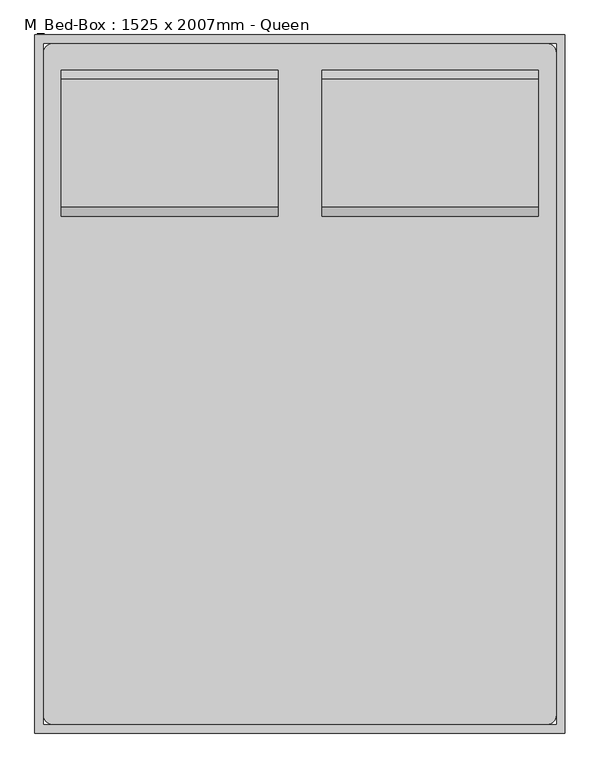
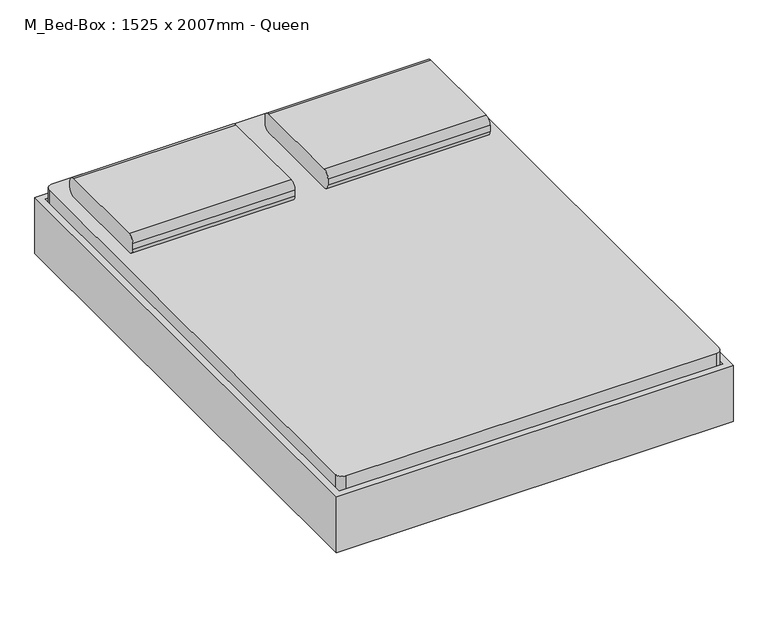
"""IFC4 building model written with IfcOpenShell, lengths in millimetres: furniture geometry, M_Bed-Box : 1525 x 2007mm - Queen."""

from ifc_helpers import new_model, si_unit, point, frame, frame_2d, origin, place, context, project, spatial, polyline, circle_curve, trimmed, segment, composite_curve, outline, extrude, source, transform, mapped, element, save
from ifc_brep_helpers import plane_surface, cylinder_surface, revolved_surface, advanced_brep


def m_bed_box_1525_x_2007mm_queen_e2603687(model_context):
    return source(origin(), model_context, "Body", "SolidModel", [
        extrude(outline(composite_curve([segment(polyline([(642.0704918, 406.4), (273.7704918, 406.4)]), True, "CONTINUOUS"), segment(trimmed(circle_curve(frame_2d((273.7704918, 431.8)), 25.4), [point((273.7704918, 406.4))], [point((248.3704918, 431.8))], False, "CARTESIAN"), True, "CONTINUOUS"), segment(polyline([(248.3704918, 431.8), (248.3704918, 457.2)]), True, "CONTINUOUS"), segment(trimmed(circle_curve(frame_2d((273.7704918, 457.2)), 25.4), [point((248.3704918, 457.2))], [point((273.7704918, 482.6))], False, "CARTESIAN"), True, "CONTINUOUS"), segment(polyline([(273.7704918, 482.6), (642.0704918, 482.6)]), True, "CONTINUOUS"), segment(trimmed(circle_curve(frame_2d((642.0704918, 457.2)), 25.4), [point((642.0704918, 482.6))], [point((667.4704918, 457.2))], False, "CARTESIAN"), True, "CONTINUOUS"), segment(polyline([(667.4704918, 457.2), (667.4704918, 431.8)]), True, "CONTINUOUS"), segment(trimmed(circle_curve(frame_2d((642.0704918, 431.8)), 25.4), [point((667.4704918, 431.8))], [point((642.0704918, 406.4))], False, "CARTESIAN"), True, "CONTINUOUS")], self_intersect=False)), frame((402.652459, 0.0, 0.0), z_axis=(1.0, 0.0, 0.0), x_axis=(0.0, 1.0, 0.0)), (0.0, 0.0, 1.0), 622.8),
        extrude(outline(composite_curve([segment(polyline([(642.0704918, 406.4), (273.7704918, 406.4)]), True, "CONTINUOUS"), segment(trimmed(circle_curve(frame_2d((273.7704918, 431.8)), 25.4), [point((273.7704918, 406.4))], [point((248.3704918, 431.8))], False, "CARTESIAN"), True, "CONTINUOUS"), segment(polyline([(248.3704918, 431.8), (248.3704918, 457.2)]), True, "CONTINUOUS"), segment(trimmed(circle_curve(frame_2d((273.7704918, 457.2)), 25.4), [point((248.3704918, 457.2))], [point((273.7704918, 482.6))], False, "CARTESIAN"), True, "CONTINUOUS"), segment(polyline([(273.7704918, 482.6), (642.0704918, 482.6)]), True, "CONTINUOUS"), segment(trimmed(circle_curve(frame_2d((642.0704918, 457.2)), 25.4), [point((642.0704918, 482.6))], [point((667.4704918, 457.2))], False, "CARTESIAN"), True, "CONTINUOUS"), segment(polyline([(667.4704918, 457.2), (667.4704918, 431.8)]), True, "CONTINUOUS"), segment(trimmed(circle_curve(frame_2d((642.0704918, 431.8)), 25.4), [point((667.4704918, 431.8))], [point((642.0704918, 406.4))], False, "CARTESIAN"), True, "CONTINUOUS")], self_intersect=False)), frame((-347.147541, 0.0, 0.0), z_axis=(1.0, 0.0, 0.0), x_axis=(0.0, 1.0, 0.0)), (0.0, 0.0, 1.0), 622.8),
        advanced_brep(
        [(-397.6231784, 515.0704918, 177.8), (-397.6231784, 438.8704918, 177.8), (-397.6231784, 438.8704918, 196.85), (-397.6231784, 515.0704918, 196.85), (-346.8231784, 515.0704918, 177.8), (-346.8231784, 438.8704918, 177.8), (-334.6869899, 438.8704918, 196.85), (-334.6869899, 515.0704918, 196.85), (-270.7523099, 515.0704918, 14.6654962), (-270.7523099, 438.8704918, 14.6654962), (-253.4871466, 438.8704918, 22.716374), (-253.4871466, 515.0704918, 22.716374), (-247.7320921, 438.8704918, 0.0), (-247.7320921, 515.0704918, 0.0), (-247.7320921, 438.8704918, 19.05), (-247.7320921, 515.0704918, 19.05), (-169.1195862, 515.0704918, 0.0), (-169.1195862, 438.8704918, 0.0), (-169.1195862, 438.8704918, 19.05), (-169.1195862, 515.0704918, 19.05), (-156.4195862, 438.8704918, 3.4029547), (-156.4195862, 515.0704918, 3.4029547), (-165.9445862, 438.8704918, 19.9007387), (-165.9445862, 515.0704918, 19.9007387), (-96.322541, 515.0704918, 38.1), (-96.322541, 438.8704918, 38.1), (-101.4269731, 438.8704918, 57.15), (-101.4269731, 515.0704918, 57.15), (774.9518216, 515.0704918, 38.1), (774.9518216, 438.8704918, 38.1), (780.0562537, 438.8704918, 57.15), (780.0562537, 515.0704918, 57.15), (835.0488669, 515.0704918, 3.4029547), (835.0488669, 438.8704918, 3.4029547), (844.5738669, 438.8704918, 19.9007387), (844.5738669, 515.0704918, 19.9007387), (847.7488669, 438.8704918, 0.0), (847.7488669, 515.0704918, 0.0), (847.7488669, 438.8704918, 19.05), (847.7488669, 515.0704918, 19.05), (926.3613728, 515.0704918, 0.0), (926.3613728, 438.8704918, 0.0), (926.3613728, 438.8704918, 19.05), (926.3613728, 515.0704918, 19.05), (949.3815906, 438.8704918, 14.6654962), (949.3815906, 515.0704918, 14.6654962), (932.1164272, 438.8704918, 22.716374), (932.1164272, 515.0704918, 22.716374), (1025.452459, 515.0704918, 177.8), (1025.452459, 438.8704918, 177.8), (1013.3162705, 438.8704918, 196.85), (1013.3162705, 515.0704918, 196.85), (1076.252459, 515.0704918, 177.8), (1076.252459, 515.0704918, 196.85), (1076.252459, 438.8704918, 196.85), (1076.252459, 438.8704918, 177.8)],
        [
            (0, 1),
            (1, 2),
            (2, 3),
            (3, 0),
            (0, 4),
            (4, 5),
            (5, 1),
            (5, 6),
            (6, 2),
            (6, 7),
            (7, 3),
            (7, 4),
            (4, 8),
            (8, 9),
            (9, 5),
            (9, 10),
            (10, 6),
            (10, 11),
            (11, 7),
            (11, 8),
            (12, 9, circle_curve(frame((-247.7320921, 438.8704918, 25.4), z_axis=(0.0, 1.0, 0.0), x_axis=(-0.906307787036649, 0.0, -0.4226182617407015)), 25.4)),
            (8, 13, circle_curve(frame((-247.7320921, 515.0704918, 25.4), z_axis=(0.0, -1.0, 0.0), x_axis=(-0.906307787036649, 0.0, -0.4226182617407015)), 25.4)),
            (13, 12),
            (14, 10, circle_curve(frame((-247.7320921, 438.8704918, 25.4), z_axis=(0.0, 1.0, 0.0), x_axis=(-0.906307787036649, 0.0, -0.4226182617407015)), 6.35)),
            (12, 14),
            (15, 11, circle_curve(frame((-247.7320921, 515.0704918, 25.4), z_axis=(0.0, 1.0, 0.0), x_axis=(-0.906307787036649, 0.0, -0.4226182617407015)), 6.35)),
            (14, 15),
            (15, 13),
            (13, 16),
            (16, 17),
            (17, 12),
            (17, 18),
            (18, 14),
            (18, 19),
            (19, 15),
            (19, 16),
            (20, 17, circle_curve(frame((-169.1195862, 438.8704918, 25.4), z_axis=(0.0, 1.0, 0.0), x_axis=(0.0, 0.0, -1.0)), 25.4)),
            (16, 21, circle_curve(frame((-169.1195862, 515.0704918, 25.4), z_axis=(0.0, -1.0, 0.0), x_axis=(0.0, 0.0, -1.0)), 25.4)),
            (21, 20),
            (22, 18, circle_curve(frame((-169.1195862, 438.8704918, 25.4), z_axis=(0.0, 1.0, 0.0), x_axis=(0.0, 0.0, -1.0)), 6.35)),
            (20, 22),
            (23, 19, circle_curve(frame((-169.1195862, 515.0704918, 25.4), z_axis=(0.0, 1.0, 0.0), x_axis=(0.0, 0.0, -1.0)), 6.35)),
            (22, 23),
            (23, 21),
            (21, 24),
            (24, 25),
            (25, 20),
            (25, 26),
            (26, 22),
            (26, 27),
            (27, 23),
            (27, 24),
            (24, 28),
            (28, 29),
            (29, 25),
            (29, 30),
            (30, 26),
            (30, 31),
            (31, 27),
            (31, 28),
            (28, 32),
            (32, 33),
            (33, 29),
            (33, 34),
            (34, 30),
            (34, 35),
            (35, 31),
            (35, 32),
            (36, 33, circle_curve(frame((847.7488669, 438.8704918, 25.4), z_axis=(0.0, 1.0, 0.0), x_axis=(-0.5000000000000463, 0.0, -0.8660254037844118)), 25.4)),
            (32, 37, circle_curve(frame((847.7488669, 515.0704918, 25.4), z_axis=(0.0, -1.0, 0.0), x_axis=(-0.5000000000000463, 0.0, -0.8660254037844118)), 25.4)),
            (37, 36),
            (38, 34, circle_curve(frame((847.7488669, 438.8704918, 25.4), z_axis=(0.0, 1.0, 0.0), x_axis=(-0.5000000000000463, 0.0, -0.8660254037844118)), 6.35)),
            (36, 38),
            (39, 35, circle_curve(frame((847.7488669, 515.0704918, 25.4), z_axis=(0.0, 1.0, 0.0), x_axis=(-0.5000000000000463, 0.0, -0.8660254037844118)), 6.35)),
            (38, 39),
            (39, 37),
            (37, 40),
            (40, 41),
            (41, 36),
            (41, 42),
            (42, 38),
            (42, 43),
            (43, 39),
            (43, 40),
            (44, 41, circle_curve(frame((926.3613728, 438.8704918, 25.4), z_axis=(0.0, 1.0, 0.0), x_axis=(0.0, 0.0, -1.0)), 25.4)),
            (40, 45, circle_curve(frame((926.3613728, 515.0704918, 25.4), z_axis=(0.0, -1.0, 0.0), x_axis=(0.0, 0.0, -1.0)), 25.4)),
            (45, 44),
            (46, 42, circle_curve(frame((926.3613728, 438.8704918, 25.4), z_axis=(0.0, 1.0, 0.0), x_axis=(0.0, 0.0, -1.0)), 6.35)),
            (44, 46),
            (47, 43, circle_curve(frame((926.3613728, 515.0704918, 25.4), z_axis=(0.0, 1.0, 0.0), x_axis=(0.0, 0.0, -1.0)), 6.35)),
            (46, 47),
            (47, 45),
            (45, 48),
            (48, 49),
            (49, 44),
            (49, 50),
            (50, 46),
            (50, 51),
            (51, 47),
            (51, 48),
            (52, 53),
            (53, 54),
            (54, 55),
            (55, 52),
            (48, 52),
            (55, 49),
            (54, 50),
            (53, 51),
        ],
        [
            plane_surface(frame((-397.6231784, 769.0704918, -152.9490627), z_axis=(-1.0, 0.0, 0.0), x_axis=(0.0, 1.0, 0.0))),
            plane_surface(frame((-397.6231784, 515.0704918, 177.8), z_axis=(0.0, 0.0, -1.0), x_axis=(1.0, 0.0, 0.0))),
            plane_surface(frame((-397.6231784, 438.8704918, 177.8), z_axis=(0.0, -1.0, 0.0), x_axis=(1.0, 0.0, 0.0))),
            plane_surface(frame((-397.6231784, 438.8704918, 196.85), z_axis=(0.0, 0.0, 1.0), x_axis=(1.0, 0.0, 0.0))),
            plane_surface(frame((-397.6231784, 515.0704918, 196.85), z_axis=(0.0, 1.0, 0.0), x_axis=(1.0, 0.0, 0.0))),
            plane_surface(frame((-346.8231784, 515.0704918, 177.8), z_axis=(-0.9063077870366485, 0.0, -0.4226182617407029), x_axis=(0.4226182617407029, 0.0, -0.9063077870366485))),
            plane_surface(frame((-346.8231784, 438.8704918, 177.8), z_axis=(0.0, -1.0, 0.0), x_axis=(0.42261826174070266, 0.0, -0.9063077870366485))),
            plane_surface(frame((-334.6869899, 438.8704918, 196.85), z_axis=(0.9063077870366486, 0.0, 0.4226182617407026), x_axis=(0.4226182617407026, 0.0, -0.9063077870366486))),
            plane_surface(frame((-334.6869899, 515.0704918, 196.85), z_axis=(0.0, 1.0, 0.0), x_axis=(0.42261826174070266, 0.0, -0.9063077870366485))),
            cylinder_surface(frame((-247.7320921, 769.0704918, 25.4), z_axis=(0.0, -1.0, 0.0), x_axis=(-0.906307787036649, 0.0, -0.4226182617407015)), 25.4),
            plane_surface(frame((-247.7320921, 438.8704918, 25.4), z_axis=(0.0, -1.0, 0.0), x_axis=(-0.906307787036649, 0.0, -0.4226182617407015))),
            revolved_surface(polyline([(-253.4871465476827, 438.8704918, 22.716374037946544), (-253.4871465476827, 515.0704918, 22.716374037946544)]), (-247.7320921, 769.0704918, 25.4), (0.0, -1.0, 0.0)),
            plane_surface(frame((-247.7320921, 515.0704918, 25.4), z_axis=(0.0, 1.0, 0.0), x_axis=(-0.906307787036649, 0.0, -0.4226182617407015))),
            plane_surface(frame((-247.7320921, 515.0704918, 0.0), z_axis=(0.0, 0.0, -1.0), x_axis=(1.0, 0.0, 0.0))),
            plane_surface(frame((-247.7320921, 438.8704918, 0.0), z_axis=(0.0, -1.0, 0.0), x_axis=(1.0, 0.0, 0.0))),
            plane_surface(frame((-247.7320921, 438.8704918, 19.05), z_axis=(0.0, 0.0, 1.0), x_axis=(1.0, 0.0, 0.0))),
            plane_surface(frame((-247.7320921, 515.0704918, 19.05), z_axis=(0.0, 1.0, 0.0), x_axis=(1.0, 0.0, 0.0))),
            cylinder_surface(frame((-169.1195862, 769.0704918, 25.4), z_axis=(0.0, -1.0, 0.0), x_axis=(0.0, 0.0, -1.0)), 25.4),
            plane_surface(frame((-169.1195862, 438.8704918, 25.4), z_axis=(0.0, -1.0, 0.0), x_axis=(0.0, 0.0, -1.0))),
            revolved_surface(polyline([(-169.1195862, 438.8704918, 19.049999999999997), (-169.1195862, 515.0704918, 19.049999999999997)]), (-169.1195862, 769.0704918, 25.4), (0.0, -1.0, 0.0)),
            plane_surface(frame((-169.1195862, 515.0704918, 25.4), z_axis=(0.0, 1.0, 0.0), x_axis=(0.0, 0.0, -1.0))),
            plane_surface(frame((-156.4195862, 515.0704918, 3.4029547), z_axis=(0.49999999999987765, 0.0, -0.8660254037845093), x_axis=(0.8660254037845093, 0.0, 0.49999999999987765))),
            plane_surface(frame((-156.4195862, 438.8704918, 3.4029547), z_axis=(0.0, -1.0, 0.0), x_axis=(0.8660254037845091, 0.0, 0.499999999999878))),
            plane_surface(frame((-165.9445862, 438.8704918, 19.9007387), z_axis=(-0.49999999999987765, 0.0, 0.8660254037845093), x_axis=(0.8660254037845093, 0.0, 0.49999999999987765))),
            plane_surface(frame((-165.9445862, 515.0704918, 19.9007387), z_axis=(0.0, 1.0000000000000002, 0.0), x_axis=(0.8660254037845089, 0.0, 0.4999999999998785))),
            plane_surface(frame((-96.322541, 515.0704918, 38.1), z_axis=(0.0, 0.0, -1.0), x_axis=(1.0, 0.0, 0.0))),
            plane_surface(frame((-96.322541, 438.8704918, 38.1), z_axis=(0.0, -1.0, 0.0), x_axis=(1.0, 0.0, 0.0))),
            plane_surface(frame((-101.4269731, 438.8704918, 57.15), z_axis=(0.0, 0.0, 1.0), x_axis=(1.0, 0.0, 0.0))),
            plane_surface(frame((-101.4269731, 515.0704918, 57.15), z_axis=(0.0, 1.0, 0.0), x_axis=(1.0, 0.0, 0.0))),
            plane_surface(frame((774.9518216, 515.0704918, 38.1), z_axis=(-0.5000000000000452, 0.0, -0.8660254037844126), x_axis=(0.8660254037844126, 0.0, -0.5000000000000452))),
            plane_surface(frame((774.9518216, 438.8704918, 38.1), z_axis=(0.0, -1.0, 0.0), x_axis=(0.8660254037844124, 0.0, -0.5000000000000455))),
            plane_surface(frame((780.0562537, 438.8704918, 57.15), z_axis=(0.5000000000000464, 0.0, 0.8660254037844118), x_axis=(0.8660254037844118, 0.0, -0.5000000000000464))),
            plane_surface(frame((780.0562537, 515.0704918, 57.15), z_axis=(0.0, 1.0000000000000002, 0.0), x_axis=(0.866025403784413, 0.0, -0.5000000000000447))),
            cylinder_surface(frame((847.7488669, 769.0704918, 25.4), z_axis=(0.0, -1.0, 0.0), x_axis=(-0.5000000000000463, 0.0, -0.8660254037844118)), 25.4),
            plane_surface(frame((847.7488669, 438.8704918, 25.4), z_axis=(0.0, -1.0000000000000002, 0.0), x_axis=(-0.5000000000000464, 0.0, -0.866025403784412))),
            revolved_surface(polyline([(844.5738668999998, 438.8704918, 19.90073868596898), (844.5738668999998, 515.0704918, 19.90073868596898)]), (847.7488669, 769.0704918, 25.4), (0.0, -1.0, 0.0)),
            plane_surface(frame((847.7488669, 515.0704918, 25.4), z_axis=(0.0, 1.0000000000000002, 0.0), x_axis=(-0.5000000000000464, 0.0, -0.866025403784412))),
            plane_surface(frame((847.7488669, 515.0704918, 0.0), z_axis=(0.0, 0.0, -1.0), x_axis=(1.0, 0.0, 0.0))),
            plane_surface(frame((847.7488669, 438.8704918, 0.0), z_axis=(0.0, -1.0, 0.0), x_axis=(1.0, 0.0, 0.0))),
            plane_surface(frame((847.7488669, 438.8704918, 19.05), z_axis=(0.0, 0.0, 1.0), x_axis=(1.0, 0.0, 0.0))),
            plane_surface(frame((847.7488669, 515.0704918, 19.05), z_axis=(0.0, 1.0, 0.0), x_axis=(1.0, 0.0, 0.0))),
            cylinder_surface(frame((926.3613728, 769.0704918, 25.4), z_axis=(0.0, -1.0, 0.0), x_axis=(0.0, 0.0, -1.0)), 25.4),
            plane_surface(frame((926.3613728, 438.8704918, 25.4), z_axis=(0.0, -1.0, 0.0), x_axis=(0.0, 0.0, -1.0))),
            revolved_surface(polyline([(926.3613728, 438.8704918, 19.049999999999997), (926.3613728, 515.0704918, 19.049999999999997)]), (926.3613728, 769.0704918, 25.4), (0.0, -1.0, 0.0)),
            plane_surface(frame((926.3613728, 515.0704918, 25.4), z_axis=(0.0, 1.0, 0.0), x_axis=(0.0, 0.0, -1.0))),
            plane_surface(frame((949.3815906, 515.0704918, 14.6654962), z_axis=(0.9063077870366805, 0.0, -0.422618261740634), x_axis=(0.422618261740634, 0.0, 0.9063077870366805))),
            plane_surface(frame((949.3815906, 438.8704918, 14.6654962), z_axis=(0.0, -1.0, 0.0), x_axis=(0.4226182617406339, 0.0, 0.9063077870366806))),
            plane_surface(frame((932.1164272, 438.8704918, 22.716374), z_axis=(-0.9063077870366808, 0.0, 0.4226182617406335), x_axis=(0.4226182617406335, 0.0, 0.9063077870366808))),
            plane_surface(frame((932.1164272, 515.0704918, 22.716374), z_axis=(0.0, 1.0, 0.0), x_axis=(0.42261826174063294, 0.0, 0.906307787036681))),
            plane_surface(frame((1076.252459, 769.0704918, -152.9490627), z_axis=(1.0, 0.0, 0.0), x_axis=(0.0, 1.0, 0.0))),
            plane_surface(frame((1025.452459, 515.0704918, 177.8), z_axis=(0.0, 0.0, -1.0), x_axis=(1.0, 0.0, 0.0))),
            plane_surface(frame((1025.452459, 438.8704918, 177.8), z_axis=(0.0, -1.0, 0.0), x_axis=(1.0, 0.0, 0.0))),
            plane_surface(frame((1013.3162705, 438.8704918, 196.85), z_axis=(0.0, 0.0, 1.0), x_axis=(1.0, 0.0, 0.0))),
            plane_surface(frame((1013.3162705, 515.0704918, 196.85), z_axis=(0.0, 1.0, 0.0), x_axis=(1.0, 0.0, 0.0))),
        ],
        [
            (0, [[1, 2, 3, 4]]),
            (1, [[-1, 5, 6, 7]]),
            (2, [[-2, -7, 8, 9]]),
            (3, [[-3, -9, 10, 11]]),
            (4, [[-4, -11, 12, -5]]),
            (5, [[-6, 13, 14, 15]]),
            (6, [[-8, -15, 16, 17]]),
            (7, [[-10, -17, 18, 19]]),
            (8, [[-12, -19, 20, -13]]),
            (9, [[21, -14, 22, 23]]),
            (10, [[24, -16, -21, 25]]),
            (11, [[26, -18, -24, 27]]),
            (12, [[-22, -20, -26, 28]]),
            (13, [[-23, 29, 30, 31]]),
            (14, [[-25, -31, 32, 33]]),
            (15, [[-27, -33, 34, 35]]),
            (16, [[-28, -35, 36, -29]]),
            (17, [[37, -30, 38, 39]]),
            (18, [[40, -32, -37, 41]]),
            (19, [[42, -34, -40, 43]]),
            (20, [[-38, -36, -42, 44]]),
            (21, [[-39, 45, 46, 47]]),
            (22, [[-41, -47, 48, 49]]),
            (23, [[-43, -49, 50, 51]]),
            (24, [[-44, -51, 52, -45]]),
            (25, [[-46, 53, 54, 55]]),
            (26, [[-48, -55, 56, 57]]),
            (27, [[-50, -57, 58, 59]]),
            (28, [[-52, -59, 60, -53]]),
            (29, [[-54, 61, 62, 63]]),
            (30, [[-56, -63, 64, 65]]),
            (31, [[-58, -65, 66, 67]]),
            (32, [[-60, -67, 68, -61]]),
            (33, [[69, -62, 70, 71]]),
            (34, [[72, -64, -69, 73]]),
            (35, [[74, -66, -72, 75]]),
            (36, [[-70, -68, -74, 76]]),
            (37, [[-71, 77, 78, 79]]),
            (38, [[-73, -79, 80, 81]]),
            (39, [[-75, -81, 82, 83]]),
            (40, [[-76, -83, 84, -77]]),
            (41, [[85, -78, 86, 87]]),
            (42, [[88, -80, -85, 89]]),
            (43, [[90, -82, -88, 91]]),
            (44, [[-86, -84, -90, 92]]),
            (45, [[-87, 93, 94, 95]]),
            (46, [[-89, -95, 96, 97]]),
            (47, [[-91, -97, 98, 99]]),
            (48, [[-92, -99, 100, -93]]),
            (49, [[101, 102, 103, 104]]),
            (50, [[-94, 105, -104, 106]]),
            (51, [[-96, -106, -103, 107]]),
            (52, [[-98, -107, -102, 108]]),
            (53, [[-100, -108, -101, -105]]),
        ],
    ),
        extrude(outline(composite_curve([segment(polyline([(-372.547541, 743.6704918), (1050.852459, 743.6704918)]), True, "CONTINUOUS"), segment(trimmed(circle_curve(frame_2d((1050.852459, 718.2704918)), 25.4), [point((1050.852459, 743.6704918))], [point((1076.252459, 718.2704918))], False, "CARTESIAN"), True, "CONTINUOUS"), segment(polyline([(1076.252459, 718.2704918), (1076.252459, -1187.1295082)]), True, "CONTINUOUS"), segment(trimmed(circle_curve(frame_2d((1050.852459, -1187.1295082)), 25.4), [point((1076.252459, -1187.1295082))], [point((1050.852459, -1212.5295082))], False, "CARTESIAN"), True, "CONTINUOUS"), segment(polyline([(1050.852459, -1212.5295082), (-372.547541, -1212.5295082)]), True, "CONTINUOUS"), segment(trimmed(circle_curve(frame_2d((-372.547541, -1187.1295082)), 25.4), [point((-372.547541, -1212.5295082))], [point((-397.947541, -1187.1295082))], False, "CARTESIAN"), True, "CONTINUOUS"), segment(polyline([(-397.947541, -1187.1295082), (-397.947541, 718.2704918)]), True, "CONTINUOUS"), segment(trimmed(circle_curve(frame_2d((-372.547541, 718.2704918)), 25.4), [point((-397.947541, 718.2704918))], [point((-372.547541, 743.6704918))], False, "CARTESIAN"), True, "CONTINUOUS")], self_intersect=False)), frame((0.0, 0.0, 203.2), z_axis=(0.0, 0.0, 1.0), x_axis=(1.0, 0.0, 0.0)), (0.0, 0.0, 1.0), 203.2),
        advanced_brep(
        [(-397.947541, -933.1295082, 196.85), (-397.947541, -933.1295082, 177.8), (-397.947541, -1009.3295082, 177.8), (-397.947541, -1009.3295082, 196.85), (-335.0113525, -933.1295082, 196.85), (-347.147541, -933.1295082, 177.8), (-347.147541, -1009.3295082, 177.8), (-335.0113525, -1009.3295082, 196.85), (-253.8115092, -933.1295082, 22.716374), (-271.0766725, -933.1295082, 14.6654962), (-271.0766725, -1009.3295082, 14.6654962), (-253.8115092, -1009.3295082, 22.716374), (-248.0564547, -933.1295082, 0.0), (-248.0564547, -933.1295082, 19.05), (-248.0564547, -1009.3295082, 0.0), (-248.0564547, -1009.3295082, 19.05), (-169.4439489, -933.1295082, 19.05), (-169.4439489, -933.1295082, 0.0), (-169.4439489, -1009.3295082, 0.0), (-169.4439489, -1009.3295082, 19.05), (-156.7439489, -933.1295082, 3.4029547), (-166.2689489, -933.1295082, 19.9007387), (-156.7439489, -1009.3295082, 3.4029547), (-166.2689489, -1009.3295082, 19.9007387), (-101.7513357, -933.1295082, 57.15), (-96.6469036, -933.1295082, 38.1), (-96.6469036, -1009.3295082, 38.1), (-101.7513357, -1009.3295082, 57.15), (780.0562537, -933.1295082, 57.15), (774.9518216, -933.1295082, 38.1), (774.9518216, -1009.3295082, 38.1), (780.0562537, -1009.3295082, 57.15), (844.5738669, -933.1295082, 19.9007387), (835.0488669, -933.1295082, 3.4029547), (835.0488669, -1009.3295082, 3.4029547), (844.5738669, -1009.3295082, 19.9007387), (847.7488669, -933.1295082, 0.0), (847.7488669, -933.1295082, 19.05), (847.7488669, -1009.3295082, 0.0), (847.7488669, -1009.3295082, 19.05), (926.3613728, -933.1295082, 19.05), (926.3613728, -933.1295082, 0.0), (926.3613728, -1009.3295082, 0.0), (926.3613728, -1009.3295082, 19.05), (949.3815906, -933.1295082, 14.6654962), (932.1164272, -933.1295082, 22.716374), (949.3815906, -1009.3295082, 14.6654962), (932.1164272, -1009.3295082, 22.716374), (1013.3162705, -933.1295082, 196.85), (1025.452459, -933.1295082, 177.8), (1025.452459, -1009.3295082, 177.8), (1013.3162705, -1009.3295082, 196.85), (1076.252459, -933.1295082, 196.85), (1076.252459, -1009.3295082, 196.85), (1076.252459, -1009.3295082, 177.8), (1076.252459, -933.1295082, 177.8)],
        [
            (0, 1),
            (1, 2),
            (2, 3),
            (3, 0),
            (0, 4),
            (4, 5),
            (5, 1),
            (5, 6),
            (6, 2),
            (6, 7),
            (7, 3),
            (7, 4),
            (4, 8),
            (8, 9),
            (9, 5),
            (9, 10),
            (10, 6),
            (10, 11),
            (11, 7),
            (11, 8),
            (12, 9, circle_curve(frame((-248.0564547, -933.1295082, 25.4), z_axis=(0.0, 1.0, 0.0), x_axis=(-0.9063077870366625, 0.0, -0.4226182617406725)), 25.4)),
            (8, 13, circle_curve(frame((-248.0564547, -933.1295082, 25.4), z_axis=(0.0, -1.0, 0.0), x_axis=(-0.9063077870366625, 0.0, -0.4226182617406725)), 6.35)),
            (13, 12),
            (14, 10, circle_curve(frame((-248.0564547, -1009.3295082, 25.4), z_axis=(0.0, 1.0, 0.0), x_axis=(-0.9063077870366625, 0.0, -0.4226182617406725)), 25.4)),
            (12, 14),
            (15, 11, circle_curve(frame((-248.0564547, -1009.3295082, 25.4), z_axis=(0.0, 1.0, 0.0), x_axis=(-0.9063077870366625, 0.0, -0.4226182617406725)), 6.35)),
            (14, 15),
            (15, 13),
            (13, 16),
            (16, 17),
            (17, 12),
            (17, 18),
            (18, 14),
            (18, 19),
            (19, 15),
            (19, 16),
            (20, 17, circle_curve(frame((-169.4439489, -933.1295082, 25.4), z_axis=(0.0, 1.0, 0.0), x_axis=(0.0, 0.0, -1.0)), 25.4)),
            (16, 21, circle_curve(frame((-169.4439489, -933.1295082, 25.4), z_axis=(0.0, -1.0, 0.0), x_axis=(0.0, 0.0, -1.0)), 6.35)),
            (21, 20),
            (22, 18, circle_curve(frame((-169.4439489, -1009.3295082, 25.4), z_axis=(0.0, 1.0, 0.0), x_axis=(0.0, 0.0, -1.0)), 25.4)),
            (20, 22),
            (23, 19, circle_curve(frame((-169.4439489, -1009.3295082, 25.4), z_axis=(0.0, 1.0, 0.0), x_axis=(0.0, 0.0, -1.0)), 6.35)),
            (22, 23),
            (23, 21),
            (21, 24),
            (24, 25),
            (25, 20),
            (25, 26),
            (26, 22),
            (26, 27),
            (27, 23),
            (27, 24),
            (24, 28),
            (28, 29),
            (29, 25),
            (29, 30),
            (30, 26),
            (30, 31),
            (31, 27),
            (31, 28),
            (28, 32),
            (32, 33),
            (33, 29),
            (33, 34),
            (34, 30),
            (34, 35),
            (35, 31),
            (35, 32),
            (36, 33, circle_curve(frame((847.7488669, -933.1295082, 25.4), z_axis=(0.0, 1.0, 0.0), x_axis=(-0.5000000000000528, 0.0, -0.8660254037844081)), 25.4)),
            (32, 37, circle_curve(frame((847.7488669, -933.1295082, 25.4), z_axis=(0.0, -1.0, 0.0), x_axis=(-0.5000000000000528, 0.0, -0.8660254037844081)), 6.35)),
            (37, 36),
            (38, 34, circle_curve(frame((847.7488669, -1009.3295082, 25.4), z_axis=(0.0, 1.0, 0.0), x_axis=(-0.5000000000000528, 0.0, -0.8660254037844081)), 25.4)),
            (36, 38),
            (39, 35, circle_curve(frame((847.7488669, -1009.3295082, 25.4), z_axis=(0.0, 1.0, 0.0), x_axis=(-0.5000000000000528, 0.0, -0.8660254037844081)), 6.35)),
            (38, 39),
            (39, 37),
            (37, 40),
            (40, 41),
            (41, 36),
            (41, 42),
            (42, 38),
            (42, 43),
            (43, 39),
            (43, 40),
            (44, 41, circle_curve(frame((926.3613728, -933.1295082, 25.4), z_axis=(0.0, 1.0, 0.0), x_axis=(0.0, 0.0, -1.0)), 25.4)),
            (40, 45, circle_curve(frame((926.3613728, -933.1295082, 25.4), z_axis=(0.0, -1.0, 0.0), x_axis=(0.0, 0.0, -1.0)), 6.35)),
            (45, 44),
            (46, 42, circle_curve(frame((926.3613728, -1009.3295082, 25.4), z_axis=(0.0, 1.0, 0.0), x_axis=(0.0, 0.0, -1.0)), 25.4)),
            (44, 46),
            (47, 43, circle_curve(frame((926.3613728, -1009.3295082, 25.4), z_axis=(0.0, 1.0, 0.0), x_axis=(0.0, 0.0, -1.0)), 6.35)),
            (46, 47),
            (47, 45),
            (45, 48),
            (48, 49),
            (49, 44),
            (49, 50),
            (50, 46),
            (50, 51),
            (51, 47),
            (51, 48),
            (52, 53),
            (53, 54),
            (54, 55),
            (55, 52),
            (48, 52),
            (55, 49),
            (54, 50),
            (53, 51),
        ],
        [
            plane_surface(frame((-397.947541, -1237.9295082, -127.5947323), z_axis=(-1.0, 0.0, 0.0), x_axis=(0.0, 1.0, 0.0))),
            plane_surface(frame((-397.947541, -933.1295082, 196.85), z_axis=(0.0, 1.0, 0.0), x_axis=(1.0, 0.0, 0.0))),
            plane_surface(frame((-397.947541, -933.1295082, 177.8), z_axis=(0.0, 0.0, -1.0), x_axis=(1.0, 0.0, 0.0))),
            plane_surface(frame((-397.947541, -1009.3295082, 177.8), z_axis=(0.0, -1.0, 0.0), x_axis=(1.0, 0.0, 0.0))),
            plane_surface(frame((-397.947541, -1009.3295082, 196.85), z_axis=(0.0, 0.0, 1.0), x_axis=(1.0, 0.0, 0.0))),
            plane_surface(frame((-335.0113525, -933.1295082, 196.85), z_axis=(0.0, 1.0, 0.0), x_axis=(0.42261826174067124, 0.0, -0.9063077870366631))),
            plane_surface(frame((-347.147541, -933.1295082, 177.8), z_axis=(-0.9063077870366631, 0.0, -0.42261826174067113), x_axis=(0.42261826174067113, 0.0, -0.9063077870366631))),
            plane_surface(frame((-347.147541, -1009.3295082, 177.8), z_axis=(0.0, -1.0, 0.0), x_axis=(0.422618261740671, 0.0, -0.9063077870366633))),
            plane_surface(frame((-335.0113525, -1009.3295082, 196.85), z_axis=(0.9063077870366631, 0.0, 0.42261826174067124), x_axis=(0.42261826174067124, 0.0, -0.9063077870366631))),
            plane_surface(frame((-248.0564547, -933.1295082, 25.4), z_axis=(0.0, 1.0, 0.0), x_axis=(-0.9063077870366625, 0.0, -0.4226182617406725))),
            cylinder_surface(frame((-248.0564547, -1237.9295082, 25.4), z_axis=(0.0, -1.0, 0.0), x_axis=(-0.9063077870366625, 0.0, -0.4226182617406725)), 25.4),
            plane_surface(frame((-248.0564547, -1009.3295082, 25.4), z_axis=(0.0, -1.0, 0.0), x_axis=(-0.9063077870366625, 0.0, -0.4226182617406725))),
            revolved_surface(polyline([(-253.81150914768278, -1009.3295082, 22.71637403794673), (-253.81150914768278, -933.1295082, 22.71637403794673)]), (-248.0564547, -1237.9295082, 25.4), (0.0, -1.0, 0.0)),
            plane_surface(frame((-248.0564547, -933.1295082, 19.05), z_axis=(0.0, 1.0, 0.0), x_axis=(1.0, 0.0, 0.0))),
            plane_surface(frame((-248.0564547, -933.1295082, 0.0), z_axis=(0.0, 0.0, -1.0), x_axis=(1.0, 0.0, 0.0))),
            plane_surface(frame((-248.0564547, -1009.3295082, 0.0), z_axis=(0.0, -1.0, 0.0), x_axis=(1.0, 0.0, 0.0))),
            plane_surface(frame((-248.0564547, -1009.3295082, 19.05), z_axis=(0.0, 0.0, 1.0), x_axis=(1.0, 0.0, 0.0))),
            plane_surface(frame((-169.4439489, -933.1295082, 25.4), z_axis=(0.0, 1.0, 0.0), x_axis=(0.0, 0.0, -1.0))),
            cylinder_surface(frame((-169.4439489, -1237.9295082, 25.4), z_axis=(0.0, -1.0, 0.0), x_axis=(0.0, 0.0, -1.0)), 25.4),
            plane_surface(frame((-169.4439489, -1009.3295082, 25.4), z_axis=(0.0, -1.0, 0.0), x_axis=(0.0, 0.0, -1.0))),
            revolved_surface(polyline([(-169.4439489, -1009.3295082, 19.049999999999997), (-169.4439489, -933.1295082, 19.049999999999997)]), (-169.4439489, -1237.9295082, 25.4), (0.0, -1.0, 0.0)),
            plane_surface(frame((-166.2689489, -933.1295082, 19.9007387), z_axis=(0.0, 1.0, 0.0), x_axis=(0.8660254037844788, 0.0, 0.49999999999993056))),
            plane_surface(frame((-156.7439489, -933.1295082, 3.4029547), z_axis=(0.4999999999999305, 0.0, -0.8660254037844788), x_axis=(0.8660254037844788, 0.0, 0.4999999999999305))),
            plane_surface(frame((-156.7439489, -1009.3295082, 3.4029547), z_axis=(0.0, -1.0, 0.0), x_axis=(0.8660254037844788, 0.0, 0.49999999999993044))),
            plane_surface(frame((-166.2689489, -1009.3295082, 19.9007387), z_axis=(-0.49999999999993033, 0.0, 0.8660254037844789), x_axis=(0.8660254037844789, 0.0, 0.49999999999993033))),
            plane_surface(frame((-101.7513357, -933.1295082, 57.15), z_axis=(0.0, 1.0, 0.0), x_axis=(1.0, 0.0, 0.0))),
            plane_surface(frame((-96.6469036, -933.1295082, 38.1), z_axis=(0.0, 0.0, -1.0), x_axis=(1.0, 0.0, 0.0))),
            plane_surface(frame((-96.6469036, -1009.3295082, 38.1), z_axis=(0.0, -1.0, 0.0), x_axis=(1.0, 0.0, 0.0))),
            plane_surface(frame((-101.7513357, -1009.3295082, 57.15), z_axis=(0.0, 0.0, 1.0), x_axis=(1.0, 0.0, 0.0))),
            plane_surface(frame((780.0562537, -933.1295082, 57.15), z_axis=(0.0, 1.0, 0.0), x_axis=(0.8660254037844092, 0.0, -0.5000000000000511))),
            plane_surface(frame((774.9518216, -933.1295082, 38.1), z_axis=(-0.5000000000000514, 0.0, -0.866025403784409), x_axis=(0.866025403784409, 0.0, -0.5000000000000514))),
            plane_surface(frame((774.9518216, -1009.3295082, 38.1), z_axis=(0.0, -1.0, 0.0), x_axis=(0.8660254037844092, 0.0, -0.5000000000000512))),
            plane_surface(frame((780.0562537, -1009.3295082, 57.15), z_axis=(0.500000000000051, 0.0, 0.8660254037844093), x_axis=(0.8660254037844093, 0.0, -0.500000000000051))),
            plane_surface(frame((847.7488669, -933.1295082, 25.4), z_axis=(0.0, 1.0000000000000002, 0.0), x_axis=(-0.500000000000053, 0.0, -0.8660254037844082))),
            cylinder_surface(frame((847.7488669, -1237.9295082, 25.4), z_axis=(0.0, -1.0, 0.0), x_axis=(-0.5000000000000528, 0.0, -0.8660254037844081)), 25.4),
            plane_surface(frame((847.7488669, -1009.3295082, 25.4), z_axis=(0.0, -1.0000000000000002, 0.0), x_axis=(-0.500000000000053, 0.0, -0.8660254037844082))),
            revolved_surface(polyline([(844.5738668999998, -1009.3295082, 19.900738685969007), (844.5738668999998, -933.1295082, 19.900738685969007)]), (847.7488669, -1237.9295082, 25.4), (0.0, -1.0, 0.0)),
            plane_surface(frame((847.7488669, -933.1295082, 19.05), z_axis=(0.0, 1.0, 0.0), x_axis=(1.0, 0.0, 0.0))),
            plane_surface(frame((847.7488669, -933.1295082, 0.0), z_axis=(0.0, 0.0, -1.0), x_axis=(1.0, 0.0, 0.0))),
            plane_surface(frame((847.7488669, -1009.3295082, 0.0), z_axis=(0.0, -1.0, 0.0), x_axis=(1.0, 0.0, 0.0))),
            plane_surface(frame((847.7488669, -1009.3295082, 19.05), z_axis=(0.0, 0.0, 1.0), x_axis=(1.0, 0.0, 0.0))),
            plane_surface(frame((926.3613728, -933.1295082, 25.4), z_axis=(0.0, 1.0, 0.0), x_axis=(0.0, 0.0, -1.0))),
            cylinder_surface(frame((926.3613728, -1237.9295082, 25.4), z_axis=(0.0, -1.0, 0.0), x_axis=(0.0, 0.0, -1.0)), 25.4),
            plane_surface(frame((926.3613728, -1009.3295082, 25.4), z_axis=(0.0, -1.0, 0.0), x_axis=(0.0, 0.0, -1.0))),
            revolved_surface(polyline([(926.3613728, -1009.3295082, 19.049999999999997), (926.3613728, -933.1295082, 19.049999999999997)]), (926.3613728, -1237.9295082, 25.4), (0.0, -1.0, 0.0)),
            plane_surface(frame((932.1164272, -933.1295082, 22.716374), z_axis=(0.0, 1.0, 0.0), x_axis=(0.42261826174053974, 0.0, 0.9063077870367244))),
            plane_surface(frame((949.3815906, -933.1295082, 14.6654962), z_axis=(0.9063077870367244, 0.0, -0.42261826174053996), x_axis=(0.42261826174053996, 0.0, 0.9063077870367244))),
            plane_surface(frame((949.3815906, -1009.3295082, 14.6654962), z_axis=(0.0, -1.0, 0.0), x_axis=(0.4226182617405396, 0.0, 0.9063077870367245))),
            plane_surface(frame((932.1164272, -1009.3295082, 22.716374), z_axis=(-0.9063077870367247, 0.0, 0.4226182617405392), x_axis=(0.4226182617405392, 0.0, 0.9063077870367247))),
            plane_surface(frame((1076.252459, -1237.9295082, -127.5947323), z_axis=(1.0, 0.0, 0.0), x_axis=(0.0, 1.0, 0.0))),
            plane_surface(frame((1013.3162705, -933.1295082, 196.85), z_axis=(0.0, 1.0, 0.0), x_axis=(1.0, 0.0, 0.0))),
            plane_surface(frame((1025.452459, -933.1295082, 177.8), z_axis=(0.0, 0.0, -1.0), x_axis=(1.0, 0.0, 0.0))),
            plane_surface(frame((1025.452459, -1009.3295082, 177.8), z_axis=(0.0, -1.0, 0.0), x_axis=(1.0, 0.0, 0.0))),
            plane_surface(frame((1013.3162705, -1009.3295082, 196.85), z_axis=(0.0, 0.0, 1.0), x_axis=(1.0, 0.0, 0.0))),
        ],
        [
            (0, [[1, 2, 3, 4]]),
            (1, [[-1, 5, 6, 7]]),
            (2, [[-2, -7, 8, 9]]),
            (3, [[-3, -9, 10, 11]]),
            (4, [[-4, -11, 12, -5]]),
            (5, [[-6, 13, 14, 15]]),
            (6, [[-8, -15, 16, 17]]),
            (7, [[-10, -17, 18, 19]]),
            (8, [[-12, -19, 20, -13]]),
            (9, [[21, -14, 22, 23]]),
            (10, [[24, -16, -21, 25]]),
            (11, [[26, -18, -24, 27]]),
            (12, [[-22, -20, -26, 28]]),
            (13, [[-23, 29, 30, 31]]),
            (14, [[-25, -31, 32, 33]]),
            (15, [[-27, -33, 34, 35]]),
            (16, [[-28, -35, 36, -29]]),
            (17, [[37, -30, 38, 39]]),
            (18, [[40, -32, -37, 41]]),
            (19, [[42, -34, -40, 43]]),
            (20, [[-38, -36, -42, 44]]),
            (21, [[-39, 45, 46, 47]]),
            (22, [[-41, -47, 48, 49]]),
            (23, [[-43, -49, 50, 51]]),
            (24, [[-44, -51, 52, -45]]),
            (25, [[-46, 53, 54, 55]]),
            (26, [[-48, -55, 56, 57]]),
            (27, [[-50, -57, 58, 59]]),
            (28, [[-52, -59, 60, -53]]),
            (29, [[-54, 61, 62, 63]]),
            (30, [[-56, -63, 64, 65]]),
            (31, [[-58, -65, 66, 67]]),
            (32, [[-60, -67, 68, -61]]),
            (33, [[69, -62, 70, 71]]),
            (34, [[72, -64, -69, 73]]),
            (35, [[74, -66, -72, 75]]),
            (36, [[-70, -68, -74, 76]]),
            (37, [[-71, 77, 78, 79]]),
            (38, [[-73, -79, 80, 81]]),
            (39, [[-75, -81, 82, 83]]),
            (40, [[-76, -83, 84, -77]]),
            (41, [[85, -78, 86, 87]]),
            (42, [[88, -80, -85, 89]]),
            (43, [[90, -82, -88, 91]]),
            (44, [[-86, -84, -90, 92]]),
            (45, [[-87, 93, 94, 95]]),
            (46, [[-89, -95, 96, 97]]),
            (47, [[-91, -97, 98, 99]]),
            (48, [[-92, -99, 100, -93]]),
            (49, [[101, 102, 103, 104]]),
            (50, [[-94, 105, -104, 106]]),
            (51, [[-96, -106, -103, 107]]),
            (52, [[-98, -107, -102, 108]]),
            (53, [[-100, -108, -101, -105]]),
        ],
    ),
        extrude(outline(polyline([(1101.652459, 769.0704918), (1101.652459, -1237.9295082), (-423.347541, -1237.9295082), (-423.347541, 769.0704918), (1101.652459, 769.0704918)]), holes=[polyline([(1076.252459, 743.6704918), (-397.947541, 743.6704918), (-397.947541, -1212.5295082), (1076.252459, -1212.5295082), (1076.252459, 743.6704918)])]), frame((0.0, 0.0, 127.0), z_axis=(0.0, 0.0, 1.0), x_axis=(1.0, 0.0, 0.0)), (0.0, 0.0, 1.0), 228.6),
    ])


if __name__ == "__main__":
    model = new_model("IFC4")
    model_context = context("Model", 3, world=origin())
    ifc_project = project(units=[si_unit("LENGTHUNIT", "METRE", prefix="MILLI")], contexts=[model_context])
    site = spatial("IfcSite", under=ifc_project)
    building = spatial("IfcBuilding", under=site)
    placement = place(None, origin())
    m_bed_box_1525_x_2007mm_queen_shape = m_bed_box_1525_x_2007mm_queen_e2603687(model_context)
    element("IfcFurniture", 1, ObjectType="M_Bed-Box : 1525 x 2007mm - Queen", at=placement, inside=building, context=model_context, shape_type="MappedRepresentation", body=[
        mapped(m_bed_box_1525_x_2007mm_queen_shape, transform((0.0, 0.0, 0.0), x_axis=(1.0, 0.0, 0.0), y_axis=(0.0, 1.0, 0.0), z_axis=(0.0, 0.0, 1.0))),
    ])
    save(model, "model.ifc")

# Revit data of these elements
# Type "M_Bed-Box : 1525 x 2007mm - Queen"
#   Length = 6' - 7.01575"
#   Width = 5' - 0.03937"
#   Frame Material = Birch
#   Mattress Material = Linen, White
#   Default Elevation = 0
# Element 1 (IfcFurniture, "M_Bed-Box : 1525 x 2007mm - Queen")
#   Materials on its faces: "Birch", "Linen, White"
# Materials
#   "Birch": class "Wood", colour RGB 224 178 126, transparency 0, Description = "Betula Alleghaniensis", Cost = 0
#   "Linen, White": class "Textile", colour RGB 247 247 239, transparency 0, Description = "Linen, white", Cost = 0
